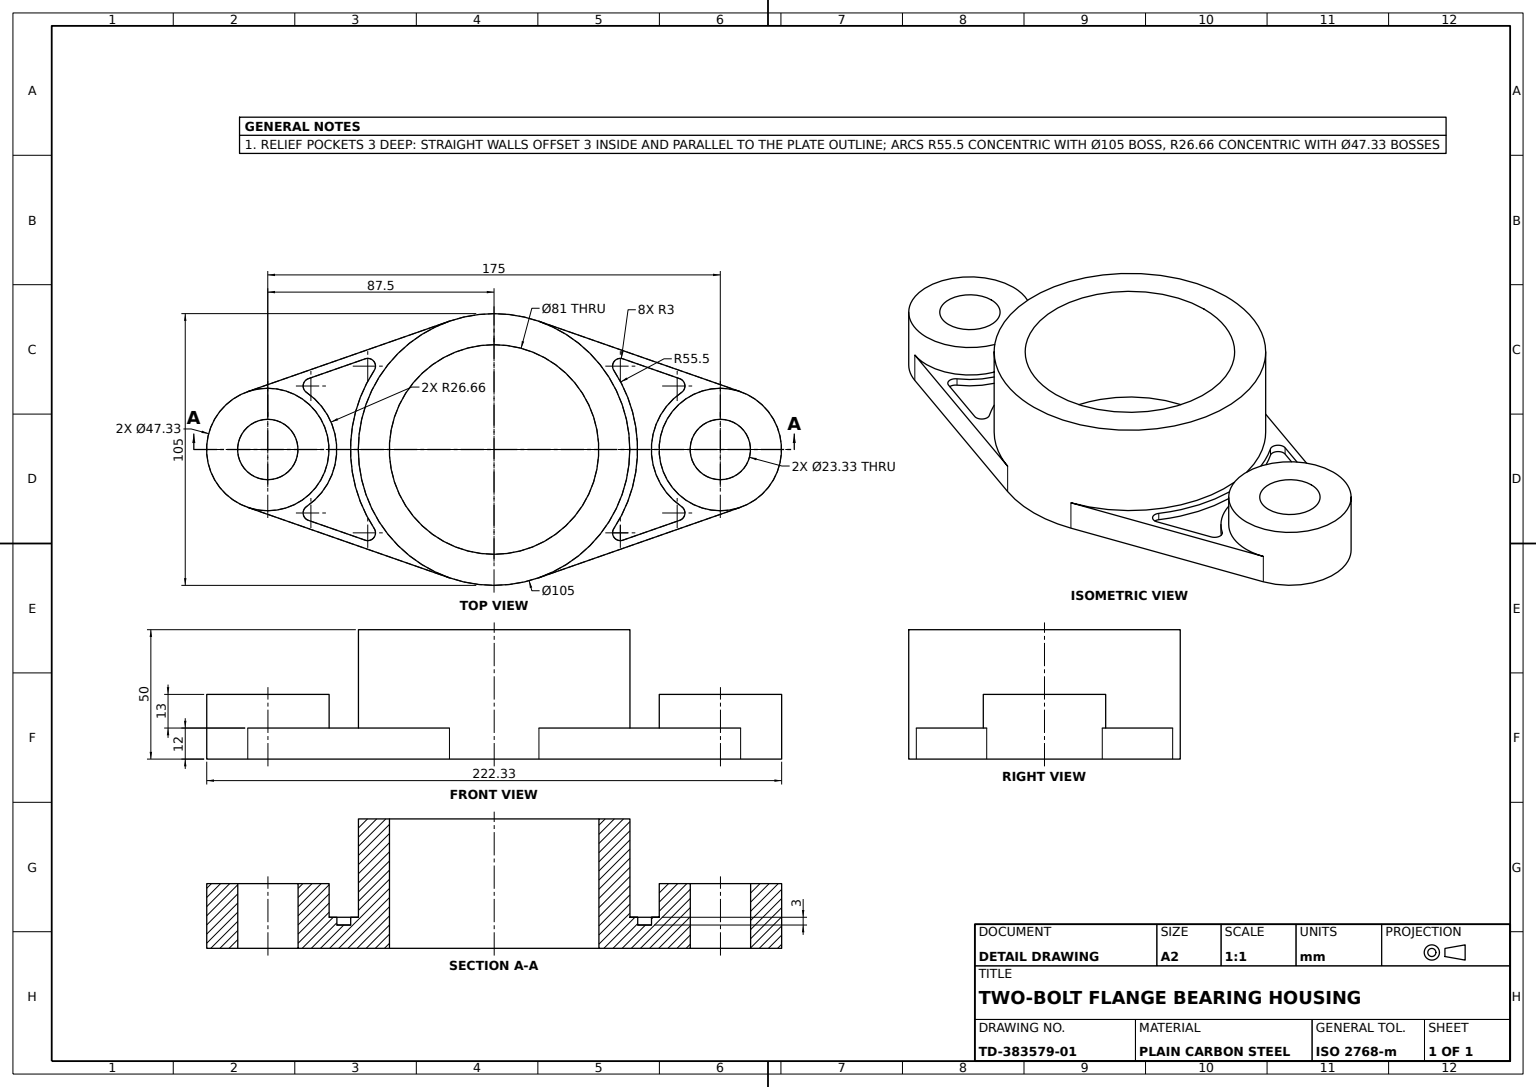
from build123d import *

# Parameters (mm, degrees)
FLANGE_PLATE_SKETCH_R       = 11.665
FLANGE_PLATE_SKETCH_R_2     = 52.5
FLANGE_PLATE_SKETCH_R_3     = 40.5
FLANGE_PLATE_DEPTH          = 12
HOUSING_BOSS_SKETCH_R       = 52.5
HOUSING_BOSS_SKETCH_R_2     = 40.5
BEARING_HOUSING_BOSS_DEPTH  = 38
BOLT_BOSS_SKETCH_R          = 23.665
BOLT_BOSS_SKETCH_R_2        = 11.665
BOLT_BOSSES_2X_DEPTH        = 13
FLANGE_RELIEF_POCKETS_DEPTH = 3


with BuildPart() as part:
    # Flange Plate Sketch → Flange Plate (new body)
    # profile 1 of 3: a face of its own
    with BuildSketch(Plane(origin=(0, 0, 0), x_dir=(1, 0, 0), z_dir=(0, 1, 0))):
        with BuildLine():
            ThreePointArc((-17.301, -49.56738241), (-52.5, 0), (-17.301, 49.56738241))
            Line((-17.301, 49.56738241), (-95.298631714, 22.343087709))
            ThreePointArc((-95.298631714, 22.343087709), (-111.165, 0), (-95.298631714, -22.343087709))
            Line((-95.298631714, -22.343087709), (-17.301, -49.56738241))
        make_face()
        with Locations(Location((-87.5, 0, 0), (0, 0, 270))):
            Circle(FLANGE_PLATE_SKETCH_R, mode=Mode.SUBTRACT)
    # profile 2 of 3: a face of its own
    with BuildSketch(Plane(origin=(0, 0, 0), x_dir=(1, 0, 0), z_dir=(0, 1, 0))):
        with BuildLine():
            Line((95.298631714, 22.343087709), (17.301, 49.56738241))
            ThreePointArc((17.301, 49.56738241), (42.805096075, 30.396936523), (52.5, 0))
            ThreePointArc((52.5, 0), (42.805096075, -30.396936523), (17.301, -49.56738241))
            Line((17.301, -49.56738241), (95.298631714, -22.343087709))
            ThreePointArc((95.298631714, -22.343087709), (111.165, 0), (95.298631714, 22.343087709))
        make_face()
        with Locations(Location((87.5, 0, 0), (0, 0, 270))):
            Circle(FLANGE_PLATE_SKETCH_R, mode=Mode.SUBTRACT)
    # profile 3 of 3: a face of its own
    with BuildSketch(Plane(origin=(0, 0, 0), x_dir=(1, 0, 0), z_dir=(0, 1, 0))):
        Circle(FLANGE_PLATE_SKETCH_R_2)
        with Locations(Location((0, 0, 0), (0, 0, 270))):
            Circle(FLANGE_PLATE_SKETCH_R_3, mode=Mode.SUBTRACT)
    extrude(amount=FLANGE_PLATE_DEPTH)

    # Housing Boss Sketch → Bearing Housing Boss (add)
    with BuildSketch(Plane(origin=(0, 12, 0), x_dir=(1, 0, 0), z_dir=(0, 1, 0))):
        with Locations(Location((0, 0, 0), (0, 0, 109.241031138))):
            Circle(HOUSING_BOSS_SKETCH_R)
        with Locations(Location((0, 0, 0), (0, 0, 270))):
            Circle(HOUSING_BOSS_SKETCH_R_2, mode=Mode.SUBTRACT)
    extrude(amount=BEARING_HOUSING_BOSS_DEPTH)

    # Bolt Boss Sketch → Bolt Bosses 2x (add)
    # profile 1 of 2: a face of its own
    with BuildSketch(Plane(origin=(0, 12, 0), x_dir=(1, 0, 0), z_dir=(0, 1, 0))):
        with Locations(Location((87.5, 0, 0), (0, 0, 70.758968862))):
            Circle(BOLT_BOSS_SKETCH_R)
        with Locations(Location((87.5, 0, 0), (0, 0, 270))):
            Circle(BOLT_BOSS_SKETCH_R_2, mode=Mode.SUBTRACT)
    # profile 2 of 2: a face of its own
    with BuildSketch(Plane(origin=(0, 12, 0), x_dir=(1, 0, 0), z_dir=(0, 1, 0))):
        with Locations(Location((-87.5, 0, 0), (0, 0, 109.241031138))):
            Circle(BOLT_BOSS_SKETCH_R)
        with Locations(Location((-87.5, 0, 0), (0, 0, 270))):
            Circle(BOLT_BOSS_SKETCH_R_2, mode=Mode.SUBTRACT)
    extrude(amount=BOLT_BOSSES_2X_DEPTH)

    # Relief Pocket Sketch → Flange Relief Pockets (cut)
    with BuildSketch(Plane(origin=(0, 12, 0), x_dir=(1, 0, 0), z_dir=(0, 1, 0))):
        with BuildLine():
            Line((71.809327621, 27.364302024), (49.82603874, 35.037349549))
            ThreePointArc((49.82603874, 35.037349549), (46.470783868, 34.048587089), (46.332927596, 30.553392944))
            ThreePointArc((46.332927596, 30.553392944), (55.5, 0), (46.332927596, -30.553392944))
            ThreePointArc((46.332927596, -30.553392944), (46.470783868, -34.048587089), (49.82603874, -35.037349549))
            Line((49.82603874, -35.037349549), (71.809327621, -27.364302024))
            ThreePointArc((71.809327621, -27.364302024), (73.795133067, -24.922702734), (72.507464694, -22.050988869))
            ThreePointArc((72.507464694, -22.050988869), (60.835, 0), (72.507464694, 22.050988869))
            ThreePointArc((72.507464694, 22.050988869), (73.795133067, 24.922702734), (71.809327621, 27.364302024))
        make_face()
        with BuildLine():
            Line((-71.809327621, -27.364302024), (-49.82603874, -35.037349549))
            ThreePointArc((-49.82603874, -35.037349549), (-46.470783868, -34.048587089), (-46.332927596, -30.553392944))
            ThreePointArc((-46.332927596, -30.553392944), (-55.5, 0), (-46.332927596, 30.553392944))
            ThreePointArc((-46.332927596, 30.553392944), (-46.470783868, 34.048587089), (-49.82603874, 35.037349549))
            Line((-49.82603874, 35.037349549), (-71.809327621, 27.364302024))
            ThreePointArc((-71.809327621, 27.364302024), (-73.795133067, 24.922702734), (-72.507464694, 22.050988869))
            ThreePointArc((-72.507464694, 22.050988869), (-60.835, 0), (-72.507464694, -22.050988869))
            ThreePointArc((-72.507464694, -22.050988869), (-73.795133067, -24.922702734), (-71.809327621, -27.364302024))
        make_face()
    extrude(amount=-FLANGE_RELIEF_POCKETS_DEPTH, mode=Mode.SUBTRACT)


solid = part.part
